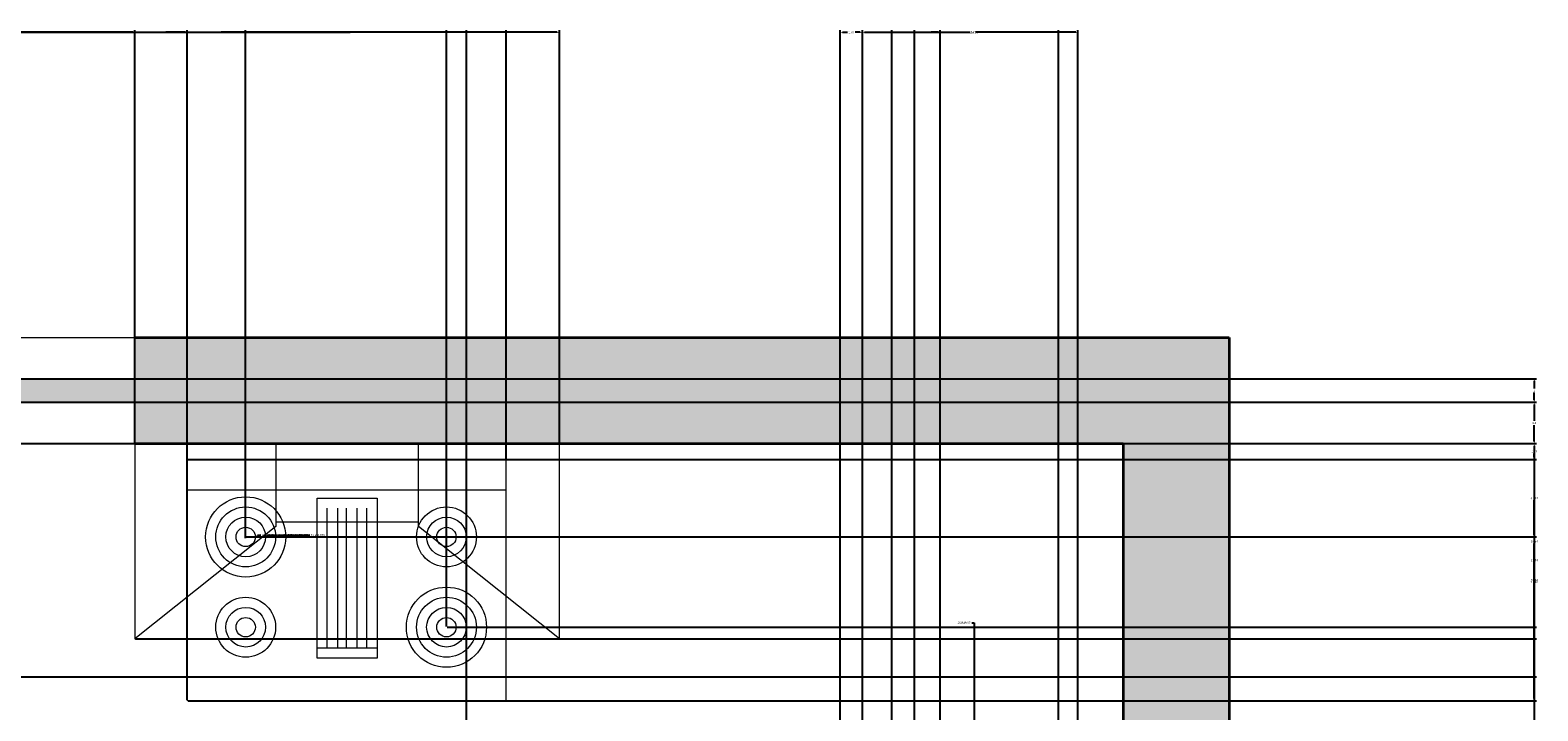
# Model space of a CAD drawing. Units: inches. Extents: x 6 to 575, y 34 to 566.
# Tile 21 of 21: x 447 to 575, y 508 to 566. Entities that reach past the tile are written whole.
import ezdxf

# ---------------------------------------------------------------- set-up
doc = ezdxf.new("R2010")
doc.units = ezdxf.units.IN
for name, color, linetype, lineweight in [('A-ANNO-DIMS', 2, 'Continuous', 18), ('A-EQPM', 2, 'Continuous', 18), ('A-GLAZ-PATT', 4, 'Continuous', 9), ('A-WALL-PATT', 251, 'Continuous', 9), ('WALLS', 7, 'Continuous', 35), ('WINDOWS', 4, 'Continuous', 20)]:
    doc.layers.add(name, color=color, linetype=linetype, lineweight=lineweight)
doc.styles.get("Standard").update_dxf_attribs({"font": 'arial.ttf'})
doc.dimstyles.get("Standard").update_dxf_attribs({"dimtxt": 0.18, "dimasz": 0.18, "dimexe": 0.18, "dimexo": 0.0625, "dimgap": 0.09, "dimtad": 0, "dimtih": 1, "dimtoh": 1, "dimdec": 4, "dimzin": 0, "dimdsep": 46, "dimtxsty": 'Standard', "dimcen": 0.09, "dimadec": 0, "dimazin": 0, "dimtfac": 1, "dimtdec": 4, "dimtofl": 0, "dimtmove": 0, "dimatfit": 3, "dimfxl": 1, "dimtolj": 1, "dimtzin": 0, "dimarcsym": 0})

# ---------------------------------------------------------------- blocks, each defined once
blk = doc.blocks.new('WIN-48IN')
for p, q in [((0, 0), (0, 9)), ((0, 0), (0, 9)), ((0, 9), (0, 0)), ((48, 0), (48, 9)), ((0, 5.5), (48, 5.5)), ((0, 3.5), (48, 3.5))]:
    blk.add_line(p, q)
blk.add_lwpolyline([(0, 9), (48, 9), (48, 0), (0, 0)], close=True)
blk = doc.blocks.new('*D53')
at = {"layer": 'A-ANNO-DIMS', "color": 0, "lineweight": -2, "transparency": 16777216}
for p, q in [((445.02, 338), (445.02, 565.81)), ((445.2, 565.63), (464.15, 565.63)), ((483.85, 565.63), (464.9, 565.63)), ((484.03, 338), (484.03, 565.81))]:
    blk.add_line(p, q, dxfattribs=at)
at = {"layer": 'A-ANNO-DIMS', "color": 0, "transparency": 16777216}
for points in [[(445.2, 565.66), (445.2, 565.6), (445.02, 565.63)], [(483.85, 565.66), (483.85, 565.6), (484.03, 565.63)]]:
    blk.add_solid(points, dxfattribs=at)
at = {"layer": 'Defpoints', "color": 0, "transparency": 16777216}
for p in [(484.03, 565.63), (445.02, 337.94), (484.03, 337.94)]:
    blk.add_point(p, dxfattribs=at)
at = {"layer": 'A-ANNO-DIMS', "color": 0, "transparency": 16777216, "insert": (464.53, 565.63), "char_height": 0.18, "attachment_point": 5}
blk.add_mtext('\\A1;39.01', dxfattribs=at)
blk = doc.blocks.new('*D152')
at = {"layer": 'A-ANNO-DIMS', "color": 0, "lineweight": -2, "transparency": 16777216}
for p, q in [((383.72, 530.8), (574.68, 530.8)), ((574.5, 530.62), (574.5, 490.26)), ((574.5, 449.53), (574.5, 489.89)), ((383.72, 449.35), (574.68, 449.35))]:
    blk.add_line(p, q, dxfattribs=at)
at = {"layer": 'A-ANNO-DIMS', "color": 0, "transparency": 16777216}
for points in [[(574.47, 530.62), (574.53, 530.62), (574.5, 530.8)], [(574.47, 449.53), (574.53, 449.53), (574.5, 449.35)]]:
    blk.add_solid(points, dxfattribs=at)
at = {"layer": 'Defpoints', "color": 0, "transparency": 16777216}
for p in [(383.66, 530.8), (574.5, 530.8), (383.66, 449.35)]:
    blk.add_point(p, dxfattribs=at)
at = {"layer": 'A-ANNO-DIMS', "color": 0, "transparency": 16777216, "insert": (574.5, 490.08), "char_height": 0.18, "attachment_point": 5}
blk.add_mtext('\\A1;81.45', dxfattribs=at)
blk = doc.blocks.new('*D153')
at = {"layer": 'A-ANNO-DIMS', "color": 0, "lineweight": -2, "transparency": 16777216}
for p, q in [((539.72, 530.8), (574.68, 530.8)), ((574.5, 530.62), (574.5, 490.92)), ((574.5, 450.86), (574.5, 490.56)), ((539.72, 450.68), (574.68, 450.68))]:
    blk.add_line(p, q, dxfattribs=at)
at = {"layer": 'A-ANNO-DIMS', "color": 0, "transparency": 16777216}
for points in [[(574.47, 530.62), (574.53, 530.62), (574.5, 530.8)], [(574.47, 450.86), (574.53, 450.86), (574.5, 450.68)]]:
    blk.add_solid(points, dxfattribs=at)
at = {"layer": 'Defpoints', "color": 0, "transparency": 16777216}
for p in [(539.66, 530.8), (574.5, 530.8), (539.66, 450.68)]:
    blk.add_point(p, dxfattribs=at)
at = {"layer": 'A-ANNO-DIMS', "color": 0, "transparency": 16777216, "insert": (574.5, 490.74), "char_height": 0.18, "attachment_point": 5}
blk.add_mtext('\\A1;80.12', dxfattribs=at)
blk = doc.blocks.new('*D155')
at = {"layer": 'A-ANNO-DIMS', "color": 0, "lineweight": -2, "transparency": 16777216}
for p, q in [((515.71, 450.74), (515.71, 565.81)), ((515.89, 565.63), (516.33, 565.63)), ((517.4, 565.63), (516.96, 565.63)), ((517.58, 452.77), (517.58, 565.81))]:
    blk.add_line(p, q, dxfattribs=at)
at = {"layer": 'A-ANNO-DIMS', "color": 0, "transparency": 16777216}
for points in [[(515.89, 565.66), (515.89, 565.6), (515.71, 565.63)], [(517.4, 565.66), (517.4, 565.6), (517.58, 565.63)]]:
    blk.add_solid(points, dxfattribs=at)
at = {"layer": 'Defpoints', "color": 0, "transparency": 16777216}
for p in [(517.58, 565.63), (517.58, 452.71), (515.71, 450.68)]:
    blk.add_point(p, dxfattribs=at)
at = {"layer": 'A-ANNO-DIMS', "color": 0, "transparency": 16777216, "insert": (516.64, 565.63), "char_height": 0.18, "attachment_point": 5}
blk.add_mtext('\\A1;1.87', dxfattribs=at)
blk = doc.blocks.new('*D157')
at = {"layer": 'A-ANNO-DIMS', "color": 0, "lineweight": -2, "transparency": 16777216}
for p, q in [((517.58, 452.77), (517.58, 565.81)), ((517.76, 565.63), (526.25, 565.63)), ((535.66, 565.63), (527.16, 565.63)), ((535.84, 452.77), (535.84, 565.81))]:
    blk.add_line(p, q, dxfattribs=at)
at = {"layer": 'A-ANNO-DIMS', "color": 0, "transparency": 16777216}
for points in [[(517.76, 565.66), (517.76, 565.6), (517.58, 565.63)], [(535.66, 565.66), (535.66, 565.6), (535.84, 565.63)]]:
    blk.add_solid(points, dxfattribs=at)
at = {"layer": 'Defpoints', "color": 0, "transparency": 16777216}
for p in [(535.84, 565.63), (517.58, 452.71), (535.84, 452.71)]:
    blk.add_point(p, dxfattribs=at)
at = {"layer": 'A-ANNO-DIMS', "color": 0, "transparency": 16777216, "insert": (526.71, 565.63), "char_height": 0.18, "attachment_point": 5}
blk.add_mtext('\\A1;18.257', dxfattribs=at)
blk = doc.blocks.new('*D160')
at = {"layer": 'A-ANNO-DIMS', "color": 0, "lineweight": -2, "transparency": 16777216}
for p, q in [((455.94, 530.86), (455.94, 565.81)), ((456.12, 565.63), (473.53, 565.63)), ((491.73, 565.63), (474.32, 565.63)), ((491.91, 530.86), (491.91, 565.81))]:
    blk.add_line(p, q, dxfattribs=at)
at = {"layer": 'A-ANNO-DIMS', "color": 0, "transparency": 16777216}
for points in [[(456.12, 565.66), (456.12, 565.6), (455.94, 565.63)], [(491.73, 565.66), (491.73, 565.6), (491.91, 565.63)]]:
    blk.add_solid(points, dxfattribs=at)
at = {"layer": 'Defpoints', "color": 0, "transparency": 16777216}
for p in [(491.91, 565.63), (455.94, 530.8), (491.91, 530.8)]:
    blk.add_point(p, dxfattribs=at)
at = {"layer": 'A-ANNO-DIMS', "color": 0, "transparency": 16777216, "insert": (473.93, 565.63), "char_height": 0.18, "attachment_point": 5}
blk.add_mtext('\\A1;35.97', dxfattribs=at)
blk = doc.blocks.new('*D161')
at = {"layer": 'A-ANNO-DIMS', "color": 0, "lineweight": -2, "transparency": 16777216}
for p, q in [((456.01, 530.8), (574.68, 530.8)), ((574.5, 530.62), (574.5, 522.71)), ((574.5, 514.44), (574.5, 522.35)), ((456.01, 514.26), (574.68, 514.26))]:
    blk.add_line(p, q, dxfattribs=at)
at = {"layer": 'A-ANNO-DIMS', "color": 0, "transparency": 16777216}
for points in [[(574.47, 530.62), (574.53, 530.62), (574.5, 530.8)], [(574.47, 514.44), (574.53, 514.44), (574.5, 514.26)]]:
    blk.add_solid(points, dxfattribs=at)
at = {"layer": 'Defpoints', "color": 0, "transparency": 16777216}
for p in [(455.94, 530.8), (455.94, 514.26), (574.5, 514.26)]:
    blk.add_point(p, dxfattribs=at)
at = {"layer": 'A-ANNO-DIMS', "color": 0, "transparency": 16777216, "insert": (574.5, 522.53), "char_height": 0.18, "attachment_point": 5}
blk.add_mtext('\\A1;16.54', dxfattribs=at)
blk = doc.blocks.new('*D162')
at = {"layer": 'A-ANNO-DIMS', "color": 0, "lineweight": -2, "transparency": 16777216}
for p, q in [((460.39, 509.1), (460.39, 565.81)), ((460.57, 565.63), (473.42, 565.63)), ((487.21, 565.63), (474.35, 565.63)), ((487.39, 529.54), (487.39, 565.81))]:
    blk.add_line(p, q, dxfattribs=at)
at = {"layer": 'A-ANNO-DIMS', "color": 0, "transparency": 16777216}
for points in [[(460.57, 565.66), (460.57, 565.6), (460.39, 565.63)], [(487.21, 565.66), (487.21, 565.6), (487.39, 565.63)]]:
    blk.add_solid(points, dxfattribs=at)
at = {"layer": 'Defpoints', "color": 0, "transparency": 16777216}
for p in [(487.39, 565.63), (487.39, 529.47), (460.39, 509.03)]:
    blk.add_point(p, dxfattribs=at)
at = {"layer": 'A-ANNO-DIMS', "color": 0, "transparency": 16777216, "insert": (473.89, 565.63), "char_height": 0.18, "attachment_point": 5}
blk.add_mtext('\\A1;26.995', dxfattribs=at)
blk = doc.blocks.new('*D163')
at = {"layer": 'A-ANNO-DIMS', "color": 0, "lineweight": -2, "transparency": 16777216}
for p, q in [((487.45, 529.47), (574.68, 529.47)), ((574.5, 529.29), (574.5, 519.44)), ((574.5, 509.21), (574.5, 519.07)), ((460.45, 509.03), (574.68, 509.03))]:
    blk.add_line(p, q, dxfattribs=at)
at = {"layer": 'A-ANNO-DIMS', "color": 0, "transparency": 16777216}
for points in [[(574.47, 529.29), (574.53, 529.29), (574.5, 529.47)], [(574.47, 509.21), (574.53, 509.21), (574.5, 509.03)]]:
    blk.add_solid(points, dxfattribs=at)
at = {"layer": 'Defpoints', "color": 0, "transparency": 16777216}
for p in [(487.39, 529.47), (574.5, 529.47), (460.39, 509.03)]:
    blk.add_point(p, dxfattribs=at)
at = {"layer": 'A-ANNO-DIMS', "color": 0, "transparency": 16777216, "insert": (574.5, 519.25), "char_height": 0.18, "attachment_point": 5}
blk.add_mtext('\\A1;20.44', dxfattribs=at)
blk = doc.blocks.new('*D164')
at = {"layer": 'A-ANNO-DIMS', "color": 0, "lineweight": -2, "transparency": 16777216}
for p, q in [((465.33, 522.96), (465.33, 565.81)), ((465.51, 565.63), (473.47, 565.63)), ((482.16, 565.63), (474.21, 565.63)), ((482.34, 515.32), (482.34, 565.81))]:
    blk.add_line(p, q, dxfattribs=at)
at = {"layer": 'A-ANNO-DIMS', "color": 0, "transparency": 16777216}
for points in [[(465.51, 565.66), (465.51, 565.6), (465.33, 565.63)], [(482.16, 565.66), (482.16, 565.6), (482.34, 565.63)]]:
    blk.add_solid(points, dxfattribs=at)
at = {"layer": 'Defpoints', "color": 0, "transparency": 16777216}
for p in [(482.34, 565.63), (465.33, 522.9), (482.34, 515.26)]:
    blk.add_point(p, dxfattribs=at)
at = {"layer": 'A-ANNO-DIMS', "color": 0, "transparency": 16777216, "insert": (473.84, 565.63), "char_height": 0.18, "attachment_point": 5}
blk.add_mtext('\\A1;17.01', dxfattribs=at)
blk = doc.blocks.new('*D165')
at = {"layer": 'A-ANNO-DIMS', "color": 0, "lineweight": -2, "transparency": 16777216}
for p, q in [((465.4, 522.9), (574.68, 522.9)), ((574.5, 522.72), (574.5, 519.26)), ((574.5, 515.44), (574.5, 518.9)), ((482.41, 515.26), (574.68, 515.26))]:
    blk.add_line(p, q, dxfattribs=at)
at = {"layer": 'A-ANNO-DIMS', "color": 0, "transparency": 16777216}
for points in [[(574.47, 522.72), (574.53, 522.72), (574.5, 522.9)], [(574.47, 515.44), (574.53, 515.44), (574.5, 515.26)]]:
    blk.add_solid(points, dxfattribs=at)
at = {"layer": 'Defpoints', "color": 0, "transparency": 16777216}
for p in [(465.33, 522.9), (482.34, 515.26), (574.5, 515.26)]:
    blk.add_point(p, dxfattribs=at)
at = {"layer": 'A-ANNO-DIMS', "color": 0, "transparency": 16777216, "insert": (574.5, 519.08), "char_height": 0.18, "attachment_point": 5}
blk.add_mtext('\\A1;7.646', dxfattribs=at)
blk = doc.blocks.new('*D166')
at = {"layer": 'A-ANNO-DIMS', "color": 0, "lineweight": -2, "transparency": 16777216}
for p, q in [((383.66, 530.86), (383.66, 565.81)), ((383.84, 565.63), (419.41, 565.63)), ((455.76, 565.63), (420.19, 565.63)), ((455.94, 530.86), (455.94, 565.81))]:
    blk.add_line(p, q, dxfattribs=at)
at = {"layer": 'A-ANNO-DIMS', "color": 0, "transparency": 16777216}
for points in [[(383.84, 565.66), (383.84, 565.6), (383.66, 565.63)], [(455.76, 565.66), (455.76, 565.6), (455.94, 565.63)]]:
    blk.add_solid(points, dxfattribs=at)
at = {"layer": 'Defpoints', "color": 0, "transparency": 16777216}
for p in [(455.94, 565.63), (383.66, 530.8), (455.94, 530.8)]:
    blk.add_point(p, dxfattribs=at)
at = {"layer": 'A-ANNO-DIMS', "color": 0, "transparency": 16777216, "insert": (419.8, 565.63), "char_height": 0.18, "attachment_point": 5}
blk.add_mtext('\\A1;72.28', dxfattribs=at)
blk = doc.blocks.new('*D167')
at = {"layer": 'A-ANNO-DIMS', "color": 0, "lineweight": -2, "transparency": 16777216}
for p, q in [((455.94, 530.86), (455.94, 565.81)), ((456.12, 565.63), (457.77, 565.63)), ((460.21, 565.63), (458.56, 565.63)), ((460.39, 529.54), (460.39, 565.81))]:
    blk.add_line(p, q, dxfattribs=at)
at = {"layer": 'A-ANNO-DIMS', "color": 0, "transparency": 16777216}
for points in [[(456.12, 565.66), (456.12, 565.6), (455.94, 565.63)], [(460.21, 565.66), (460.21, 565.6), (460.39, 565.63)]]:
    blk.add_solid(points, dxfattribs=at)
at = {"layer": 'Defpoints', "color": 0, "transparency": 16777216}
for p in [(460.39, 565.63), (455.94, 530.8), (460.39, 529.47)]:
    blk.add_point(p, dxfattribs=at)
at = {"layer": 'A-ANNO-DIMS', "color": 0, "transparency": 16777216, "insert": (458.17, 565.63), "char_height": 0.18, "attachment_point": 5}
blk.add_mtext('\\A1;4.447', dxfattribs=at)
blk = doc.blocks.new('*D168')
at = {"layer": 'A-ANNO-DIMS', "color": 0, "lineweight": -2, "transparency": 16777216}
for p, q in [((456.01, 530.8), (574.68, 530.8)), ((574.5, 530.62), (574.5, 530.32)), ((460.45, 529.47), (574.68, 529.47)), ((574.5, 529.65), (574.5, 529.96))]:
    blk.add_line(p, q, dxfattribs=at)
at = {"layer": 'A-ANNO-DIMS', "color": 0, "transparency": 16777216}
for points in [[(574.47, 530.62), (574.53, 530.62), (574.5, 530.8)], [(574.47, 529.65), (574.53, 529.65), (574.5, 529.47)]]:
    blk.add_solid(points, dxfattribs=at)
at = {"layer": 'Defpoints', "color": 0, "transparency": 16777216}
for p in [(455.94, 530.8), (460.39, 529.47), (574.5, 529.47)]:
    blk.add_point(p, dxfattribs=at)
at = {"layer": 'A-ANNO-DIMS', "color": 0, "transparency": 16777216, "insert": (574.5, 530.14), "char_height": 0.18, "attachment_point": 5}
blk.add_mtext('\\A1;1.33', dxfattribs=at)
blk = doc.blocks.new('*D169')
at = {"layer": 'A-ANNO-DIMS', "color": 0, "lineweight": -2, "transparency": 16777216}
for p, q in [((460.39, 529.54), (460.39, 565.81)), ((460.57, 565.63), (462.46, 565.63)), ((465.15, 565.63), (463.26, 565.63)), ((465.33, 522.96), (465.33, 565.81))]:
    blk.add_line(p, q, dxfattribs=at)
at = {"layer": 'A-ANNO-DIMS', "color": 0, "transparency": 16777216}
for points in [[(460.57, 565.66), (460.57, 565.6), (460.39, 565.63)], [(465.15, 565.66), (465.15, 565.6), (465.33, 565.63)]]:
    blk.add_solid(points, dxfattribs=at)
at = {"layer": 'Defpoints', "color": 0, "transparency": 16777216}
for p in [(465.33, 565.63), (460.39, 529.47), (465.33, 522.9)]:
    blk.add_point(p, dxfattribs=at)
at = {"layer": 'A-ANNO-DIMS', "color": 0, "transparency": 16777216, "insert": (462.86, 565.63), "char_height": 0.18, "attachment_point": 5}
blk.add_mtext('\\A1;4.943', dxfattribs=at)
blk = doc.blocks.new('*D170')
at = {"layer": 'A-ANNO-DIMS', "color": 0, "lineweight": -2, "transparency": 16777216}
for p, q in [((460.45, 529.47), (574.68, 529.47)), ((574.5, 529.29), (574.5, 526.37)), ((574.5, 523.08), (574.5, 526.01)), ((465.4, 522.9), (574.68, 522.9))]:
    blk.add_line(p, q, dxfattribs=at)
at = {"layer": 'A-ANNO-DIMS', "color": 0, "transparency": 16777216}
for points in [[(574.47, 529.29), (574.53, 529.29), (574.5, 529.47)], [(574.47, 523.08), (574.53, 523.08), (574.5, 522.9)]]:
    blk.add_solid(points, dxfattribs=at)
at = {"layer": 'Defpoints', "color": 0, "transparency": 16777216}
for p in [(460.39, 529.47), (465.33, 522.9), (574.5, 522.9)]:
    blk.add_point(p, dxfattribs=at)
at = {"layer": 'A-ANNO-DIMS', "color": 0, "transparency": 16777216, "insert": (574.5, 526.19), "char_height": 0.18, "attachment_point": 5}
blk.add_mtext('\\A1;6.573', dxfattribs=at)
blk = doc.blocks.new('*D171')
at = {"layer": 'A-ANNO-DIMS', "color": 0, "lineweight": -2, "transparency": 16777216}
for p, q in [((520.07, 477.64), (520.07, 565.81)), ((520.25, 565.63), (526.67, 565.63)), ((534.01, 565.63), (527.58, 565.63)), ((534.19, 477.64), (534.19, 565.81))]:
    blk.add_line(p, q, dxfattribs=at)
at = {"layer": 'A-ANNO-DIMS', "color": 0, "transparency": 16777216}
for points in [[(520.25, 565.66), (520.25, 565.6), (520.07, 565.63)], [(534.01, 565.66), (534.01, 565.6), (534.19, 565.63)]]:
    blk.add_solid(points, dxfattribs=at)
at = {"layer": 'Defpoints', "color": 0, "transparency": 16777216}
for p in [(534.19, 565.63), (520.07, 477.57), (534.19, 477.58)]:
    blk.add_point(p, dxfattribs=at)
at = {"layer": 'A-ANNO-DIMS', "color": 0, "transparency": 16777216, "insert": (527.13, 565.63), "char_height": 0.18, "attachment_point": 5}
blk.add_mtext('\\A1;14.117', dxfattribs=at)
blk = doc.blocks.new('*D173')
at = {"layer": 'A-ANNO-DIMS', "color": 0, "lineweight": -2, "transparency": 16777216}
for p, q in [((521.99, 466.78), (521.99, 565.81)), ((522.17, 565.63), (522.75, 565.63)), ((523.99, 565.63), (523.4, 565.63)), ((524.17, 466.78), (524.17, 565.81))]:
    blk.add_line(p, q, dxfattribs=at)
at = {"layer": 'A-ANNO-DIMS', "color": 0, "transparency": 16777216}
for points in [[(522.17, 565.66), (522.17, 565.6), (521.99, 565.63)], [(523.99, 565.66), (523.99, 565.6), (524.17, 565.63)]]:
    blk.add_solid(points, dxfattribs=at)
at = {"layer": 'Defpoints', "color": 0, "transparency": 16777216}
for p in [(524.17, 565.63), (521.99, 466.72), (524.17, 466.72)]:
    blk.add_point(p, dxfattribs=at)
at = {"layer": 'A-ANNO-DIMS', "color": 0, "transparency": 16777216, "insert": (523.08, 565.63), "char_height": 0.18, "attachment_point": 5}
blk.add_mtext('\\A1;2.18', dxfattribs=at)
blk = doc.blocks.new('*D191')
at = {"layer": 'A-ANNO-DIMS', "color": 0, "lineweight": -2, "transparency": 16777216}
for p, q in [((374.72, 530.8), (574.68, 530.8)), ((574.5, 530.62), (574.5, 521.11)), ((574.5, 511.24), (574.5, 520.75)), ((353.8, 511.06), (574.68, 511.06))]:
    blk.add_line(p, q, dxfattribs=at)
at = {"layer": 'A-ANNO-DIMS', "color": 0, "transparency": 16777216}
for points in [[(574.47, 530.62), (574.53, 530.62), (574.5, 530.8)], [(574.47, 511.24), (574.53, 511.24), (574.5, 511.06)]]:
    blk.add_solid(points, dxfattribs=at)
at = {"layer": 'Defpoints', "color": 0, "transparency": 16777216}
for p in [(374.66, 530.8), (353.73, 511.06), (574.5, 511.06)]:
    blk.add_point(p, dxfattribs=at)
at = {"layer": 'A-ANNO-DIMS', "color": 0, "transparency": 16777216, "insert": (574.5, 520.93), "char_height": 0.18, "attachment_point": 5}
blk.add_mtext('\\A1;19.74', dxfattribs=at)
blk = doc.blocks.new('*D217')
at = {"layer": 'A-ANNO-DIMS', "color": 0, "lineweight": -2, "transparency": 16777216}
for p, q in [((408.01, 534.3), (574.68, 534.3)), ((574.5, 534.12), (574.5, 532.73)), ((574.5, 530.98), (574.5, 532.37)), ((408.01, 530.8), (574.68, 530.8))]:
    blk.add_line(p, q, dxfattribs=at)
at = {"layer": 'A-ANNO-DIMS', "color": 0, "transparency": 16777216}
for points in [[(574.47, 534.12), (574.53, 534.12), (574.5, 534.3)], [(574.47, 530.98), (574.53, 530.98), (574.5, 530.8)]]:
    blk.add_solid(points, dxfattribs=at)
at = {"layer": 'Defpoints', "color": 0, "transparency": 16777216}
for p in [(407.94, 534.3), (574.5, 534.3), (407.94, 530.8)]:
    blk.add_point(p, dxfattribs=at)
at = {"layer": 'A-ANNO-DIMS', "color": 0, "transparency": 16777216, "insert": (574.5, 532.55), "char_height": 0.18, "attachment_point": 5}
blk.add_mtext('\\A1;3.5', dxfattribs=at)
blk = doc.blocks.new('*D218')
at = {"layer": 'A-ANNO-DIMS', "color": 0, "lineweight": -2, "transparency": 16777216}
for p, q in [((408.01, 536.3), (574.68, 536.3)), ((574.5, 536.12), (574.5, 535.48)), ((408.01, 534.3), (574.68, 534.3)), ((574.5, 534.48), (574.5, 535.12))]:
    blk.add_line(p, q, dxfattribs=at)
at = {"layer": 'A-ANNO-DIMS', "color": 0, "transparency": 16777216}
for points in [[(574.47, 536.12), (574.53, 536.12), (574.5, 536.3)], [(574.47, 534.48), (574.53, 534.48), (574.5, 534.3)]]:
    blk.add_solid(points, dxfattribs=at)
at = {"layer": 'Defpoints', "color": 0, "transparency": 16777216}
for p in [(407.94, 536.3), (574.5, 536.3), (407.94, 534.3)]:
    blk.add_point(p, dxfattribs=at)
at = {"layer": 'A-ANNO-DIMS', "color": 0, "transparency": 16777216, "insert": (574.5, 535.3), "char_height": 0.18, "attachment_point": 5}
blk.add_mtext('\\A1;2', dxfattribs=at)
blk = doc.blocks.new('*D227')
at = {"layer": 'A-ANNO-DIMS', "color": 0, "lineweight": -2, "transparency": 16777216}
for p, q in [((526.86, 515.63), (527.04, 515.63)), ((527.04, 515.63), (527.1, 485.83)), ((527.12, 435.68), (527.3, 435.68)), ((527.21, 435.59), (527.21, 435.77))]:
    blk.add_line(p, q, dxfattribs=at)
at = {"layer": 'A-ANNO-DIMS', "color": 0, "transparency": 16777216}
blk.add_solid([(527.13, 485.83), (527.07, 485.83), (527.1, 485.65)], dxfattribs=at)
at = {"layer": 'Defpoints', "color": 0, "transparency": 16777216}
for p in [(527.1, 485.65), (527.21, 435.68)]:
    blk.add_point(p, dxfattribs=at)
at = {"layer": 'A-ANNO-DIMS', "color": 0, "transparency": 16777216, "insert": (526.19, 515.63), "char_height": 0.18, "attachment_point": 5}
blk.add_mtext('\\A1;2X R49.97', dxfattribs=at)
blk = doc.blocks.new('*D246')
at = {"layer": 'A-ANNO-DIMS', "color": 0, "lineweight": -2, "transparency": 16777216}
for p, q in [((465.24, 522.9), (465.42, 522.9)), ((465.33, 522.81), (465.33, 522.99)), ((470.76, 523.06), (468.91, 523.01))]:
    blk.add_line(p, q, dxfattribs=at)
at = {"layer": 'A-ANNO-DIMS', "color": 0, "transparency": 16777216}
blk.add_solid([(468.91, 523.04), (468.91, 522.98), (468.73, 523)], dxfattribs=at)
at = {"layer": 'Defpoints', "color": 0, "transparency": 16777216}
for p in [(461.94, 522.8), (468.73, 523)]:
    blk.add_point(p, dxfattribs=at)
at = {"layer": 'A-ANNO-DIMS', "color": 0, "transparency": 16777216, "insert": (471.44, 523.06), "char_height": 0.18, "attachment_point": 5}
blk.add_mtext('\\A1;2X ∅6.788', dxfattribs=at)
blk = doc.blocks.new('*D247')
at = {"layer": 'A-ANNO-DIMS', "color": 0, "lineweight": -2, "transparency": 16777216}
for p, q in [((465.24, 522.9), (465.42, 522.9)), ((465.33, 522.81), (465.33, 522.99)), ((469.39, 523.06), (468.05, 523.01))]:
    blk.add_line(p, q, dxfattribs=at)
at = {"layer": 'A-ANNO-DIMS', "color": 0, "transparency": 16777216}
blk.add_solid([(468.05, 523.04), (468.05, 522.98), (467.87, 523)], dxfattribs=at)
at = {"layer": 'Defpoints', "color": 0, "transparency": 16777216}
for p in [(462.8, 522.8), (467.87, 523)]:
    blk.add_point(p, dxfattribs=at)
at = {"layer": 'A-ANNO-DIMS', "color": 0, "transparency": 16777216, "insert": (470.05, 523.06), "char_height": 0.18, "attachment_point": 5}
blk.add_mtext('\\A1;4X ∅5.071', dxfattribs=at)
blk = doc.blocks.new('*D248')
at = {"layer": 'A-ANNO-DIMS', "color": 0, "lineweight": -2, "transparency": 16777216}
for p, q in [((465.24, 522.9), (465.42, 522.9)), ((465.33, 522.81), (465.33, 522.99)), ((468.01, 523.06), (467.19, 523.01))]:
    blk.add_line(p, q, dxfattribs=at)
at = {"layer": 'A-ANNO-DIMS', "color": 0, "transparency": 16777216}
blk.add_solid([(467.19, 523.04), (467.19, 522.98), (467.01, 523)], dxfattribs=at)
at = {"layer": 'Defpoints', "color": 0, "transparency": 16777216}
for p in [(463.66, 522.8), (467.01, 523)]:
    blk.add_point(p, dxfattribs=at)
at = {"layer": 'A-ANNO-DIMS', "color": 0, "transparency": 16777216, "insert": (468.7, 523.06), "char_height": 0.18, "attachment_point": 5}
blk.add_mtext('\\A1;4X ∅3.355', dxfattribs=at)
blk = doc.blocks.new('*D249')
at = {"layer": 'A-ANNO-DIMS', "color": 0, "lineweight": -2, "transparency": 16777216}
for p, q in [((465.24, 522.9), (465.42, 522.9)), ((465.33, 522.81), (465.33, 522.99)), ((466.63, 523.06), (466.33, 523.02))]:
    blk.add_line(p, q, dxfattribs=at)
at = {"layer": 'A-ANNO-DIMS', "color": 0, "transparency": 16777216}
blk.add_solid([(466.32, 523.05), (466.33, 522.99), (466.15, 523)], dxfattribs=at)
at = {"layer": 'Defpoints', "color": 0, "transparency": 16777216}
for p in [(464.52, 522.8), (466.15, 523)]:
    blk.add_point(p, dxfattribs=at)
at = {"layer": 'A-ANNO-DIMS', "color": 0, "transparency": 16777216, "insert": (467.25, 523.06), "char_height": 0.18, "attachment_point": 5}
blk.add_mtext('\\A1;4X ∅1.64', dxfattribs=at)

msp = doc.modelspace()

# ---------------------------------------------------------------- hatches: boundary and pattern name
at = {"layer": 'A-GLAZ-PATT'}
h = msp.add_hatch(color=256, dxfattribs=at)
h.dxf.hatch_style = 1
h.paths.add_polyline_path([(36.1586, 224.801), (38.1586, 224.801), (38.1586, 272.801), (36.1586, 272.801)])
h.paths.add_polyline_path([(167.6586, 207.301), (167.6586, 209.301), (71.6586, 209.301), (71.6586, 207.301)])
h.paths.add_polyline_path([(264.6586, 219.301), (264.6586, 221.301), (246.6586, 221.301), (246.6586, 219.301)])
h.paths.add_polyline_path([(316.6586, 221.301), (316.6586, 219.301), (334.6586, 219.301), (334.6586, 221.301)])
h.paths.add_polyline_path([(515.6586, 207.301), (515.6586, 209.301), (407.6586, 209.301), (407.6586, 207.301)])
h.paths.add_polyline_path([(543.1586, 270.801), (545.1586, 270.801), (545.1586, 366.801), (543.1586, 366.801)])
h.paths.add_polyline_path([(407.9436, 536.301), (407.9436, 534.301), (455.9436, 534.301), (455.9436, 536.301)])
h.paths.add_polyline_path([(272.6586, 536.301), (272.6586, 534.301), (320.6586, 534.301), (320.6586, 536.301)])
at = {"layer": 'A-WALL-PATT'}
h = msp.add_hatch(color=256, dxfattribs=at)
h.dxf.hatch_style = 1
h.paths.add_polyline_path([(160.6586, 539.801), (32.6586, 539.801), (32.6586, 272.801), (41.6586, 272.801), (41.6586, 286.0643), (41.6586, 358.0764), (41.6586, 379.0637), (41.6586, 407.7709), (41.6194, 407.7709), (41.6194, 431.801), (82.8918, 431.801), (82.8918, 440.801), (65.6494, 440.801), (65.6494, 440.7732), (41.6194, 440.7732), (41.6194, 515.5941), (41.6586, 530.801), (117.6586, 530.801), (117.6586, 474.801), (120.6068, 474.801), (121.6586, 474.801), (121.6586, 530.801), (137.4275, 530.801), (137.4275, 530.8356), (141.2505, 530.8356), (160.6586, 530.801)])
h.paths.add_polyline_path([(71.6586, 212.801), (41.6586, 212.801), (41.6586, 224.801), (32.6586, 224.801), (32.6586, 203.801), (71.6586, 203.801)])
h.paths.add_polyline_path([(206.6586, 215.801), (246.6586, 215.801), (246.6586, 224.801), (206.6586, 224.801), (206.6586, 230.801), (201.8157, 230.801), (197.6586, 230.801), (197.6586, 212.801), (167.6586, 212.801), (167.6586, 203.801), (206.6586, 203.801)])
h.paths.add_polyline_path([(383.6586, 224.801), (334.6586, 224.801), (334.6586, 215.801), (374.6586, 215.801), (374.6586, 203.801), (384.0753, 203.801), (407.6586, 203.801), (407.6586, 212.801), (383.6586, 212.801)])
h.paths.add_polyline_path([(548.6586, 270.801), (539.6586, 270.801), (539.6586, 212.801), (515.6586, 212.801), (515.6586, 203.801), (548.6586, 203.801)])
h.paths.add_polyline_path([(548.6586, 412.801), (545.7108, 412.801), (539.6586, 412.801), (539.6586, 382.801), (433.708, 382.801), (433.708, 378.801), (539.6586, 378.801), (539.6586, 366.801), (548.6586, 366.801)])
h.paths.add_polyline_path([(548.6586, 539.801), (455.9436, 539.801), (455.9436, 530.801), (539.6586, 530.801), (539.6586, 440.801), (548.6586, 440.801)])
h.paths.add_polyline_path([(407.9436, 539.801), (362.6586, 539.801), (362.6586, 530.801), (374.6586, 530.801), (374.6586, 452.801), (354.6586, 452.801), (354.6586, 448.801), (374.6586, 448.801), (374.6586, 278.801), (383.6586, 278.801), (383.6586, 530.801), (407.9436, 530.801)])
h.paths.add_polyline_path([(338.6586, 539.801), (320.6586, 539.801), (320.6586, 530.801), (322.6586, 530.801), (322.6586, 448.801), (326.6586, 448.801), (326.6586, 530.801), (338.6586, 530.801)])
h.paths.add_polyline_path([(272.6586, 539.801), (184.6586, 539.801), (184.6586, 530.801), (197.6586, 530.801), (197.6586, 440.801), (176.6714, 440.801), (121.6586, 440.801), (121.6586, 446.801), (117.6586, 446.801), (117.6586, 440.801), (111.6586, 440.801), (111.6586, 431.801), (197.6586, 431.801), (197.6586, 407.7709), (197.6586, 276.801), (206.6586, 276.801), (206.6586, 530.801), (272.6586, 530.801)])

# ---------------------------------------------------------------- linework, layer by layer
at = {"layer": 'A-EQPM'}
for points in [[(455.9436, 530.801), (455.9436, 514.2608), (491.9106, 514.2608), (491.9106, 530.801)], [(467.8806, 530.801), (467.8806, 523.7792), (455.9436, 514.2608)], [(491.9106, 514.2608), (479.9736, 523.7792), (479.9736, 530.801)], [(460.3907, 526.9), (487.3855, 526.9)], [(472.2497, 513.4806), (472.2497, 525.3396)], [(473.1079, 525.3396), (473.1079, 513.4806)], [(473.8881, 513.4806), (473.8881, 525.3396)], [(474.7463, 525.3396), (474.7463, 513.4806)], [(475.6045, 513.4806), (475.6045, 525.3396)], [(467.8806, 524.1693), (479.9736, 524.1693)], [(476.4627, 513.4806), (471.3915, 513.4806)]]:
    msp.add_lwpolyline(points, dxfattribs=at)
for points in [[(487.3855, 529.4747), (487.3855, 509.0335), (460.3907, 509.0335), (460.3907, 529.4747)], [(476.4627, 526.1978), (476.4627, 512.6224), (471.3915, 512.6224), (471.3915, 526.1978)]]:
    msp.add_lwpolyline(points, close=True, dxfattribs=at)
for centre, radius in [((465.3335, 522.9019), 3.3939), ((465.3335, 522.9019), 2.5356), ((482.3425, 522.9019), 2.5356), ((465.3335, 522.9019), 1.6774), ((465.3335, 522.9019), 0.8192), ((482.3425, 522.9019), 1.6774), ((482.3425, 522.9019), 0.8192), ((482.3425, 515.2557), 3.3939), ((465.3335, 515.2557), 2.5356), ((482.3425, 515.2557), 2.5356), ((465.3335, 515.2557), 1.6774), ((465.3335, 515.2557), 0.8192), ((482.3425, 515.2557), 1.6774), ((482.3425, 515.2557), 0.8192)]:
    msp.add_circle(centre, radius, dxfattribs=at)
at = {"layer": 'WALLS'}
for p, q in [((455.9436, 539.801), (548.6586, 539.801)), ((548.6586, 539.801), (548.6586, 440.801)), ((455.9436, 530.801), (539.6586, 530.801)), ((467.6586, 530.801), (539.6586, 530.801)), ((539.6586, 530.801), (539.6586, 440.801))]:
    msp.add_line(p, q, dxfattribs=at)

# ---------------------------------------------------------------- block references
at = {"layer": 'WINDOWS'}
msp.add_blockref('WIN-48IN', (407.9439, 530.801), dxfattribs=at)

# ---------------------------------------------------------------- dimensions: what is measured, and where the dimension line sits
at = {"layer": 'A-ANNO-DIMS'}
for base, p1, p2, override, picture, middle in [((455.94359, 565.63098), (383.65864, 530.80098), (455.94359, 530.80098), {"dimdec": 2, "dimlfac": 1, "dimrnd": 0, "dimzin": 0, "dimdsep": 46, "dimlunit": 2}, '*D166', (419.80112, 565.63098)), ((484.0307, 565.631), (445.0208, 337.9397), (484.0307, 337.9397), {"dimdec": 2, "dimlfac": 1, "dimrnd": 0, "dimzin": 0, "dimdsep": 46, "dimlunit": 2}, '*D53', (464.5257, 565.631)), ((491.9106, 565.631), (455.9436, 530.801), (491.9106, 530.801), {"dimdec": 2, "dimlfac": 1, "dimrnd": 0, "dimzin": 0, "dimdsep": 46, "dimlunit": 2}, '*D160', (473.9271, 565.631)), ((460.3907, 565.631), (455.9436, 530.801), (460.3907, 529.4747), {"dimdec": 3, "dimlfac": 1, "dimrnd": 0, "dimzin": 0, "dimdsep": 46, "dimlunit": 2}, '*D167', (458.1671, 565.631)), ((487.3855, 565.631), (460.3907, 509.0335), (487.3855, 529.4747), {"dimdec": 3, "dimlfac": 1, "dimrnd": 0, "dimzin": 0, "dimdsep": 46, "dimlunit": 2}, '*D162', (473.8881, 565.631)), ((465.3335, 565.631), (460.3907, 529.4747), (465.3335, 522.9019), {"dimdec": 3, "dimlfac": 1, "dimrnd": 0, "dimzin": 0, "dimdsep": 46, "dimlunit": 2}, '*D169', (462.8621, 565.631)), ((482.3425, 565.631), (465.3335, 522.9019), (482.3425, 515.2557), {"dimdec": 2, "dimlfac": 1, "dimrnd": 0, "dimzin": 0, "dimdsep": 46, "dimlunit": 2}, '*D164', (473.838, 565.631)), ((517.5791, 565.631), (515.7066, 450.6781), (517.5791, 452.7066), {"dimdec": 2, "dimlfac": 1, "dimrnd": 0, "dimzin": 0, "dimdsep": 46, "dimlunit": 2}, '*D155', (516.6429, 565.631)), ((535.8357, 565.631), (517.5791, 452.7066), (535.8357, 452.7066), {"dimdec": 3, "dimlfac": 1, "dimrnd": 0, "dimzin": 0, "dimdsep": 46, "dimlunit": 2}, '*D157', (526.7074, 565.631)), ((534.186, 565.631), (520.0692, 477.5739), (534.186, 477.5801), {"dimdec": 3, "dimlfac": 1, "dimrnd": 0, "dimzin": 0, "dimdsep": 46, "dimlunit": 2}, '*D171', (527.1276, 565.631)), ((524.1707, 565.631), (521.9861, 466.7194), (524.1707, 466.7194), {"dimdec": 2, "dimlfac": 1, "dimrnd": 0, "dimzin": 0, "dimdsep": 46, "dimlunit": 2}, '*D173', (523.0784, 565.631))]:
    dim = msp.add_linear_dim(base=base, p1=p1, p2=p2, dimstyle='Standard', override=override, dxfattribs=at)
    dim.commit()
    dim.dimension.update_dxf_attribs({"geometry": picture, "text_midpoint": middle})
for base, p1, p2, override, picture, middle in [((574.4958, 536.301), (407.9436, 534.301), (407.9436, 536.301), {"dimdec": 0, "dimlfac": 1, "dimrnd": 0, "dimzin": 0, "dimdsep": 46, "dimlunit": 2}, '*D218', (574.4958, 535.301)), ((574.4958, 534.301), (407.9436, 530.801), (407.9436, 534.301), {"dimdec": 1, "dimlfac": 1, "dimrnd": 0, "dimzin": 0, "dimdsep": 46, "dimlunit": 2}, '*D217', (574.4958, 532.551)), ((574.4958, 511.0628), (374.6586, 530.801), (353.7344, 511.0628), {"dimdec": 2, "dimlfac": 1, "dimrnd": 0, "dimzin": 0, "dimdsep": 46, "dimlunit": 2}, '*D191', (574.4958, 520.9319)), ((574.4958, 530.801), (383.6586, 449.3517), (383.6586, 530.801), {"dimdec": 2, "dimlfac": 1, "dimrnd": 0, "dimzin": 0, "dimdsep": 46, "dimlunit": 2}, '*D152', (574.4958, 490.0764)), ((574.4958, 514.2608), (455.9436, 530.801), (455.9436, 514.2608), {"dimdec": 2, "dimlfac": 1, "dimrnd": 0, "dimzin": 0, "dimdsep": 46, "dimlunit": 2}, '*D161', (574.4958, 522.5309)), ((574.4958, 529.4747), (455.9436, 530.801), (460.3907, 529.4747), {"dimdec": 2, "dimlfac": 1, "dimrnd": 0, "dimzin": 0, "dimdsep": 46, "dimlunit": 2}, '*D168', (574.4958, 530.1378)), ((574.4958, 530.801), (539.6586, 450.6781), (539.6586, 530.801), {"dimdec": 2, "dimlfac": 1, "dimrnd": 0, "dimzin": 0, "dimdsep": 46, "dimlunit": 2}, '*D153', (574.4958, 490.7395)), ((574.4958, 529.4747), (460.3907, 509.0335), (487.3855, 529.4747), {"dimdec": 2, "dimlfac": 1, "dimrnd": 0, "dimzin": 0, "dimdsep": 46, "dimlunit": 2}, '*D163', (574.4958, 519.2541)), ((574.4958, 522.9019), (460.3907, 529.4747), (465.3335, 522.9019), {"dimdec": 3, "dimlfac": 1, "dimrnd": 0, "dimzin": 0, "dimdsep": 46, "dimlunit": 2}, '*D170', (574.4958, 526.1883)), ((574.4958, 515.2557), (465.3335, 522.9019), (482.3425, 515.2557), {"dimdec": 3, "dimlfac": 1, "dimrnd": 0, "dimzin": 0, "dimdsep": 46, "dimlunit": 2}, '*D165', (574.4958, 519.0788))]:
    dim = msp.add_linear_dim(base=base, p1=p1, p2=p2, angle=90, dimstyle='Standard', override=override, dxfattribs=at)
    dim.commit()
    dim.dimension.update_dxf_attribs({"geometry": picture, "text_midpoint": middle})
for p1, p2, text, override, picture, middle in [((461.9411, 522.8039), (468.726, 522.9999), '2X <>', {"dimdec": 3, "dimlfac": 1, "dimrnd": 0, "dimzin": 0, "dimdsep": 46, "dimlunit": 2}, '*D246', (470.7614, 523.0587)), ((462.7998, 522.8032), (467.8673, 523.0007), '4X <>', {"dimdec": 3, "dimlfac": 1, "dimrnd": 0, "dimzin": 0, "dimdsep": 46, "dimlunit": 2}, '*D247', (469.3875, 523.0599)), ((463.6592, 522.8003), (467.0079, 523.0035), '4X <>', {"dimdec": 3, "dimlfac": 1, "dimrnd": 0, "dimzin": 0, "dimdsep": 46, "dimlunit": 2}, '*D248', (468.0125, 523.0645)), ((464.5202, 522.8042), (466.1469, 522.9996), '4X <>', {"dimdec": 2, "dimlfac": 1, "dimrnd": 0, "dimzin": 0, "dimdsep": 46, "dimlunit": 2}, '*D249', (466.6349, 523.0583))]:
    dim = msp.add_diameter_dim_2p(p1=p1, p2=p2, text=text, dimstyle='Standard', override=override, dxfattribs=at)
    dim.commit()
    dim.dimension.update_dxf_attribs({"geometry": picture, "text_midpoint": middle, "dimtype": 163})
dim = msp.add_radius_dim(center=(527.2056, 435.6757), mpoint=(527.103, 485.6471), text='2X <>', dimstyle='Standard', override={"dimdec": 2, "dimlfac": 1, "dimrnd": 0, "dimzin": 0, "dimdsep": 46, "dimlunit": 2}, dxfattribs=at)
dim.commit()
dim.dimension.update_dxf_attribs({"geometry": '*D227', "text_midpoint": (526.1867, 515.6299), "dimtype": 164})

doc.saveas('drawing.dxf')
